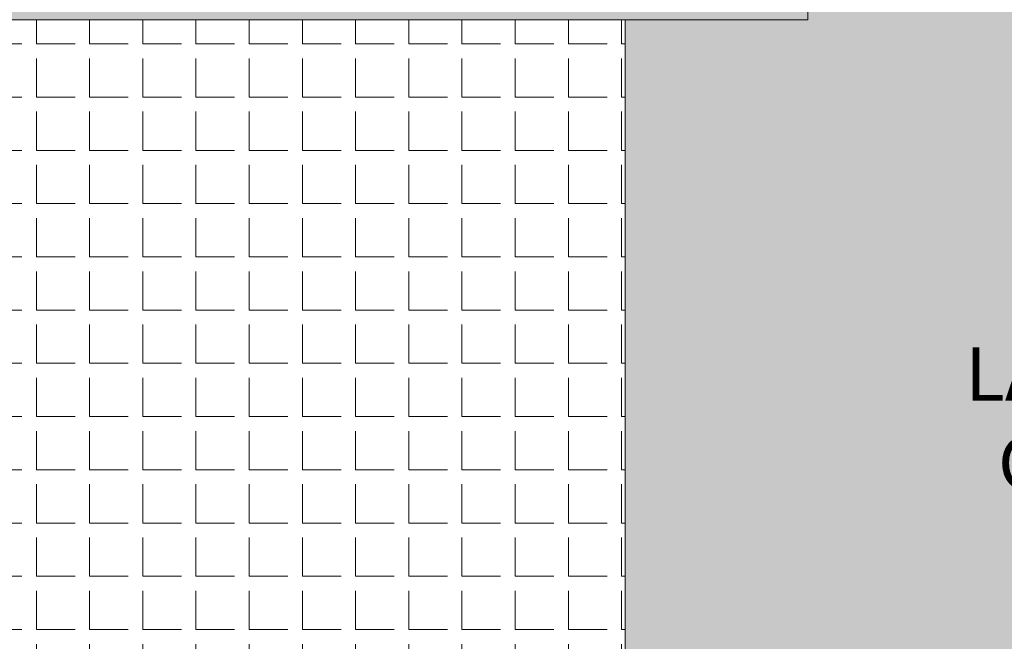
# Model space of a CAD drawing. Units: inches. Extents: x 84 to 1044, y -280 to 906.
# Tile 20 of 105: x 571 to 700, y -50 to 31. Entities that reach past the tile are written whole.
import ezdxf

# ---------------------------------------------------------------- set-up
doc = ezdxf.new("R2010")
doc.units = ezdxf.units.IN
for name, color, linetype, lineweight in [('A-AREA-IDEN', 7, 'Continuous', 13), ('A-STAIRCASE', 144, 'Continuous', 18), ('L-HRDS', 32, 'Continuous', 18)]:
    doc.layers.add(name, color=color, linetype=linetype, lineweight=lineweight)
for name, color, linetype, lineweight, true_color in [('A-FLOR-STRS-PATT', 35, 'Continuous', 9, 0x947764), ('L-HRDS-PATT', 23, 'Continuous', 9, 0xc2877b), ('L-PLNT-PATT', 9, 'Continuous', 9, 0xafd9aa)]:
    doc.layers.add(name, color=color, linetype=linetype, lineweight=lineweight, true_color=true_color)
doc.styles.add('1-100DIM', font='txt', dxfattribs={"height": 0.3})

msp = doc.modelspace()

# ---------------------------------------------------------------- hatches: boundary and pattern name
at = {"layer": 'A-FLOR-STRS-PATT', "transparency": 33554567}
h = msp.add_hatch(color=256, dxfattribs=at)
h.dxf.hatch_style = 1
h.paths.add_polyline_path([(650.074, 91.12), (638.074, 91.12), (638.074, 67.12), (455.074, 67.12), (455.074, 55.12), (650.074, 55.12)], flags=17)
h.paths.add_polyline_path([(662.074, 91.12), (650.074, 91.12), (650.074, 55.12), (455.074, 55.12), (455.074, 43.12), (662.074, 43.12)])
h.paths.add_polyline_path([(674.074, 91.12), (671.074, 91.12), (662.074, 91.12), (662.074, 43.12), (455.074, 43.12), (455.074, 31.12), (674.074, 31.12)])
h.paths.add_polyline_path([(227.179, 151.12), (203.179, 151.12), (143.179, 151.12), (143.179, 139.12), (227.179, 139.12)])
h.paths.add_polyline_path([(227.179, 139.12), (143.179, 139.12), (143.179, 127.12), (227.179, 127.12)])
h.paths.add_polyline_path([(203.179, 271.12), (143.179, 271.12), (143.179, 259.12), (203.179, 259.12)])
h.paths.add_polyline_path([(203.179, 259.12), (143.179, 259.12), (143.179, 247.12), (203.179, 247.12)])
h.paths.add_polyline_path([(203.179, 769.12), (143.179, 769.12), (143.179, 757.12), (203.179, 757.12)])
h.paths.add_polyline_path([(203.179, 757.12), (143.179, 757.12), (143.179, 745.12), (203.179, 745.12)])
h.paths.add_polyline_path([(434.074, 847.12), (422.074, 847.12), (422.074, 769.12), (434.074, 769.12)])
h.paths.add_polyline_path([(422.074, 847.12), (410.074, 847.12), (410.074, 769.12), (422.074, 769.12)])
at = {"layer": 'L-HRDS-PATT', "transparency": 33554567}
h = msp.add_hatch(dxfattribs=at)
h.set_pattern_fill('ANGLE', color=256)
h.set_pattern_definition([(0, (0, 0), (0, 6.985), [5.08, -1.905]), (90, (0, 0), (-6.985, 4e-16), [5.08, -1.905])])
h.paths.add_polyline_path([(650.074, 31.12), (504.574, 31.12), (504.574, -112.88), (504.574, -121.88), (624.574, -121.88), (624.574, -112.88), (650.074, -112.88)])
at = {"layer": 'L-PLNT-PATT', "transparency": 33554597}
h = msp.add_hatch(color=256, dxfattribs=at)
h.dxf.hatch_style = 1
h.paths.add_polyline_path([(791.074, 31.12), (791.074, 91.12), (743.074, 91.12), (674.074, 91.12), (674.074, 31.12), (650.074, 31.12), (650.074, -112.88), (983.074, -112.88), (983.074, -64.88), (791.074, -64.88)])

# ---------------------------------------------------------------- linework, layer by layer
at = {"layer": 'A-STAIRCASE'}
msp.add_lwpolyline([(674.074, 91.12), (674.074, 31.12), (455.074, 31.12)], dxfattribs=at)
at = {"layer": 'L-HRDS'}
msp.add_line((650.074, 31.12), (650.074, -112.88), dxfattribs=at)

# ---------------------------------------------------------------- texts
at = {"layer": 'A-AREA-IDEN', "insert": (694.748, -11.871), "char_height": 7, "attachment_point": 1, "style": '1-100DIM'}
msp.add_mtext_dynamic_manual_height_columns('{\\f@Malgun Gothic|b0|i0|c0|p34;LANDSCAPE\\P  GARDEN}', width=58.97918, gutter_width=15.851, heights=[0], dxfattribs=at)

doc.saveas('drawing.dxf')
